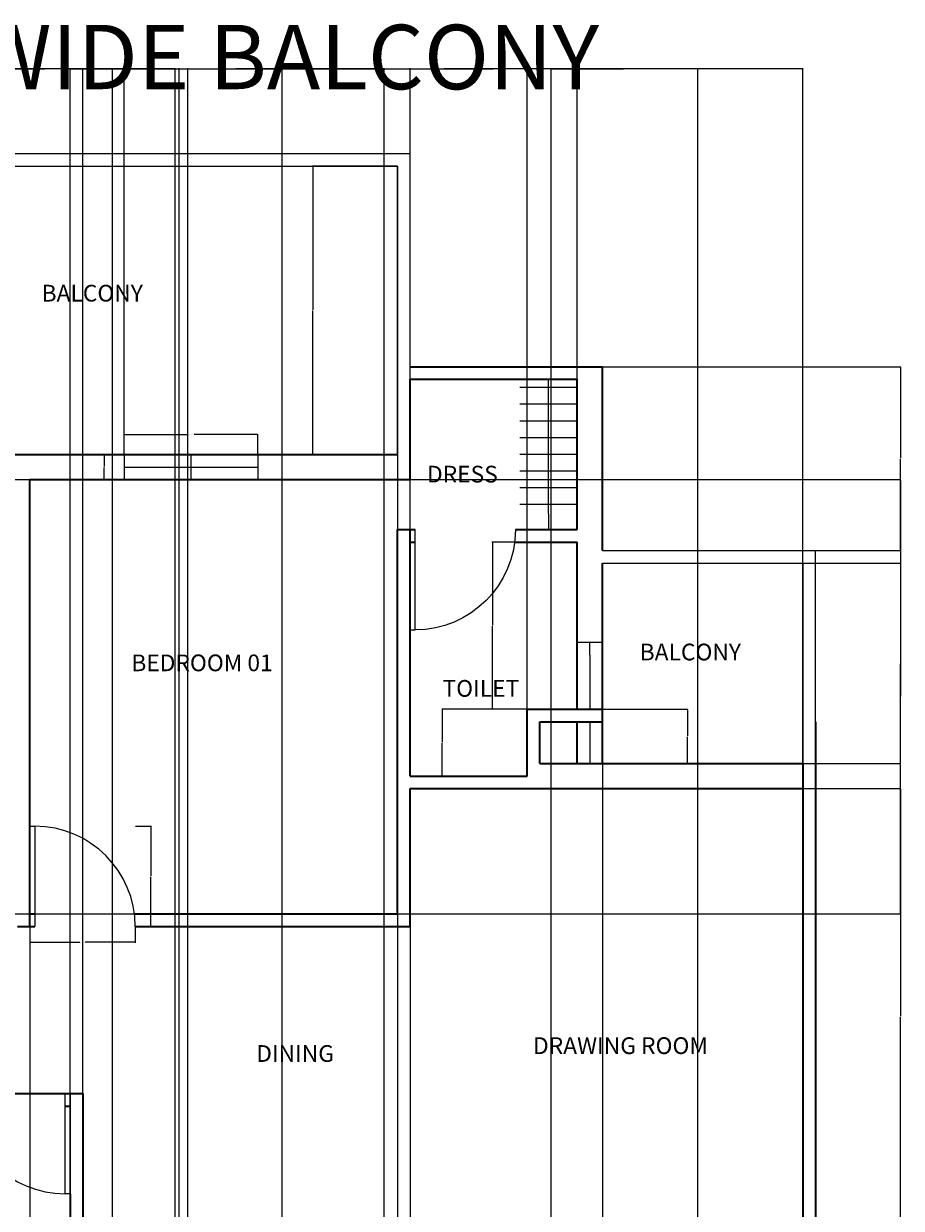
# Model space of a CAD drawing. Units: inches. Extents: x -83 to 475, y -99 to 539.
# Tile 3 of 3: x 160 to 475, y 114 to 539. Entities that reach past the tile are written whole.
import ezdxf

# ---------------------------------------------------------------- set-up
doc = ezdxf.new("R2010")
doc.units = ezdxf.units.IN
doc.header["$LTSCALE"] = 0.5
doc.header["$MEASUREMENT"] = 0
for name, color, linetype, lineweight in [('A-ANNO-DIMS', 2, 'Continuous', 18), ('A-ANNO-TEXT', 7, 'Continuous', 25), ('A-AREA-IDEN', 7, 'Continuous', 18), ('A-DOOR', 3, 'Continuous', 18), ('A-FURN', 8, 'Continuous', 13), ('A-GLAZ', 4, 'Continuous', 18), ('A-WALL', 7, 'Continuous', 35), ('A-WALL-PRPT', 7, 'Continuous', 25)]:
    doc.layers.add(name, color=color, linetype=linetype, lineweight=lineweight)
doc.styles.get("Standard").update_dxf_attribs({"font": 'arial.ttf'})
doc.dimstyles.get("Standard").update_dxf_attribs({"dimtxt": 0.18, "dimasz": 0.18, "dimexe": 0.18, "dimexo": 0.0625, "dimgap": 0.09, "dimtad": 0, "dimtih": 1, "dimtoh": 1, "dimdec": 4, "dimzin": 0, "dimdsep": 46, "dimtxsty": 'Standard', "dimcen": 0.09, "dimadec": 0, "dimazin": 0, "dimtfac": 1, "dimtdec": 4, "dimtofl": 0, "dimtmove": 0, "dimatfit": 3, "dimfxl": 1, "dimtolj": 1, "dimtzin": 0, "dimarcsym": 0})

# ---------------------------------------------------------------- blocks, each defined once
blk = doc.blocks.new('DOOR-SWING-36')
blk.add_lwpolyline([(1.78, 0), (0, 0), (0, 36.03), (1.78, 36.03)], close=True)
blk.add_arc((1.78, 0), 36, 0, 90)
blk = doc.blocks.new('WIN-48-TWO-LIGHT')
for p, q in [((0, 9), (0, 0)), ((24, 9), (24, 0)), ((48, 9), (48, 0)), ((0, 4.5), (48, 4.5))]:
    blk.add_line(p, q)
blk = doc.blocks.new('WIN-24')
for p, q in [((9, 24), (0, 24)), ((4.5, 19.41), (4.5, 24)), ((4.5, 19.41), (4.5, 0)), ((9, 0), (0, 0))]:
    blk.add_line(p, q)
blk = doc.blocks.new('WARDROBE-RAIL-48')
for p, q in [((2.64, 20.32), (2.64, 0)), ((8.64, 20.32), (8.64, 0)), ((14.64, 20.32), (14.64, 0)), ((20.64, 20.32), (20.64, 0)), ((26.64, 20.32), (26.64, 0)), ((32.64, 20.32), (32.64, 0)), ((38.64, 20.32), (38.64, 0)), ((44.64, 20.32), (44.64, 0)), ((48, 10.3), (0, 10.3))]:
    blk.add_line(p, q)
blk = doc.blocks.new('*D6')
at = {"layer": 'A-ANNO-DIMS', "color": 0, "lineweight": -2, "transparency": 16777216}
for p, q in [((162.04, 215.05), (162.04, 209.27)), ((199.82, 215.05), (199.82, 209.27)), ((162.22, 209.45), (180, 209.45)), ((199.64, 209.45), (181.87, 209.45))]:
    blk.add_line(p, q, dxfattribs=at)
at = {"layer": 'A-ANNO-DIMS', "color": 0, "transparency": 16777216}
for points in [[(162.22, 209.48), (162.22, 209.42), (162.04, 209.45)], [(199.64, 209.48), (199.64, 209.42), (199.82, 209.45)]]:
    blk.add_solid(points, dxfattribs=at)
at = {"layer": 'Defpoints', "color": 0, "transparency": 16777216}
for p in [(162.04, 215.11), (199.82, 215.11), (199.82, 209.45)]:
    blk.add_point(p, dxfattribs=at)
at = {"layer": 'A-ANNO-DIMS', "color": 0, "transparency": 16777216, "insert": (180.93, 209.45), "char_height": 0.18, "attachment_point": 5}
blk.add_mtext('\\A1;DOOR 38 TYP.', dxfattribs=at)
blk = doc.blocks.new('*D7')
at = {"layer": 'A-ANNO-DIMS', "color": 0, "lineweight": -2, "transparency": 16777216}
for p, q in [((199.89, 251.14), (205.67, 251.14)), ((205.49, 250.96), (205.49, 233.31)), ((205.49, 215.29), (205.49, 232.95)), ((199.89, 215.11), (205.67, 215.11))]:
    blk.add_line(p, q, dxfattribs=at)
at = {"layer": 'A-ANNO-DIMS', "color": 0, "transparency": 16777216}
for points in [[(205.46, 250.96), (205.52, 250.96), (205.49, 251.14)], [(205.46, 215.29), (205.52, 215.29), (205.49, 215.11)]]:
    blk.add_solid(points, dxfattribs=at)
at = {"layer": 'Defpoints', "color": 0, "transparency": 16777216}
for p in [(199.82, 251.14), (205.49, 251.14), (199.82, 215.11)]:
    blk.add_point(p, dxfattribs=at)
at = {"layer": 'A-ANNO-DIMS', "color": 0, "transparency": 16777216, "insert": (205.49, 233.13), "char_height": 0.18, "attachment_point": 5}
blk.add_mtext('\\A1;36 TYP.', dxfattribs=at)
blk = doc.blocks.new('*D8')
at = {"layer": 'A-ANNO-DIMS', "color": 0, "lineweight": -2, "transparency": 16777216}
for p, q in [((195.82, 384.62), (195.82, 391.94)), ((196, 391.76), (218.71, 391.76)), ((243.64, 391.76), (220.94, 391.76)), ((243.82, 384.62), (243.82, 391.94))]:
    blk.add_line(p, q, dxfattribs=at)
at = {"layer": 'A-ANNO-DIMS', "color": 0, "transparency": 16777216}
for points in [[(196, 391.79), (196, 391.73), (195.82, 391.76)], [(243.64, 391.79), (243.64, 391.73), (243.82, 391.76)]]:
    blk.add_solid(points, dxfattribs=at)
at = {"layer": 'Defpoints', "color": 0, "transparency": 16777216}
for p in [(243.82, 391.76), (195.82, 384.56), (243.82, 384.56)]:
    blk.add_point(p, dxfattribs=at)
at = {"layer": 'A-ANNO-DIMS', "color": 0, "transparency": 16777216, "insert": (219.82, 391.76), "char_height": 0.18, "attachment_point": 5}
blk.add_mtext('\\A1;WINDOW 48 TYP.', dxfattribs=at)
blk = doc.blocks.new('*D9')
at = {"layer": 'A-ANNO-DIMS', "color": 0, "lineweight": -2, "transparency": 16777216}
for p, q in [((195.76, 384.56), (188.44, 384.56)), ((188.62, 384.38), (188.62, 380.24)), ((188.62, 375.74), (188.62, 379.88)), ((195.76, 375.56), (188.44, 375.56))]:
    blk.add_line(p, q, dxfattribs=at)
at = {"layer": 'A-ANNO-DIMS', "color": 0, "transparency": 16777216}
for points in [[(188.59, 384.38), (188.65, 384.38), (188.62, 384.56)], [(188.59, 375.74), (188.65, 375.74), (188.62, 375.56)]]:
    blk.add_solid(points, dxfattribs=at)
at = {"layer": 'Defpoints', "color": 0, "transparency": 16777216}
for p in [(188.62, 384.56), (195.82, 384.56), (195.82, 375.56)]:
    blk.add_point(p, dxfattribs=at)
at = {"layer": 'A-ANNO-DIMS', "color": 0, "transparency": 16777216, "insert": (188.62, 380.06), "char_height": 0.18, "attachment_point": 5}
blk.add_mtext('\\A1;9 TYP.', dxfattribs=at)
blk = doc.blocks.new('*D15')
at = {"layer": 'A-ANNO-DIMS', "color": 0, "lineweight": -2, "transparency": 16777216}
for p, q in [((73.48, 492.61), (-83.14, 492.61)), ((-82.96, 492.43), (-82.96, 212.3)), ((-82.96, -68.21), (-82.96, 211.93)), ((214.1, -68.39), (-83.14, -68.39))]:
    blk.add_line(p, q, dxfattribs=at)
at = {"layer": 'A-ANNO-DIMS', "color": 0, "transparency": 16777216}
for points in [[(-82.99, 492.43), (-82.93, 492.43), (-82.96, 492.61)], [(-82.99, -68.21), (-82.93, -68.21), (-82.96, -68.39)]]:
    blk.add_solid(points, dxfattribs=at)
at = {"layer": 'Defpoints', "color": 0, "transparency": 16777216}
for p in [(-82.96, 492.61), (73.54, 492.61), (214.16, -68.39)]:
    blk.add_point(p, dxfattribs=at)
at = {"layer": 'A-ANNO-DIMS', "color": 0, "transparency": 16777216, "insert": (-82.96, 212.11), "char_height": 0.18, "attachment_point": 5}
blk.add_mtext('\\A1;561', dxfattribs=at)
blk = doc.blocks.new('*D16')
at = {"layer": 'A-ANNO-DIMS', "color": 0, "lineweight": -2, "transparency": 16777216}
for p, q in [((78.04, 488.05), (78.04, -99.07)), ((294.04, 488.05), (294.04, -99.07)), ((78.22, -98.89), (185.75, -98.89)), ((293.86, -98.89), (186.33, -98.89))]:
    blk.add_line(p, q, dxfattribs=at)
at = {"layer": 'A-ANNO-DIMS', "color": 0, "transparency": 16777216}
for points in [[(78.22, -98.86), (78.22, -98.92), (78.04, -98.89)], [(293.86, -98.86), (293.86, -98.92), (294.04, -98.89)]]:
    blk.add_solid(points, dxfattribs=at)
at = {"layer": 'Defpoints', "color": 0, "transparency": 16777216}
for p in [(78.04, 488.11), (294.04, 488.11), (294.04, -98.89)]:
    blk.add_point(p, dxfattribs=at)
at = {"layer": 'A-ANNO-DIMS', "color": 0, "transparency": 16777216, "insert": (186.04, -98.89), "char_height": 0.18, "attachment_point": 5}
blk.add_mtext('\\A1;216', dxfattribs=at)
blk = doc.blocks.new('*D17')
at = {"layer": 'A-ANNO-DIMS', "color": 0, "lineweight": -2, "transparency": 16777216}
for p, q in [((293.98, 488.11), (263.36, 488.11)), ((263.54, 487.93), (263.54, 436.55)), ((263.54, 384.79), (263.54, 436.18)), ((293.98, 384.61), (263.36, 384.61))]:
    blk.add_line(p, q, dxfattribs=at)
at = {"layer": 'A-ANNO-DIMS', "color": 0, "transparency": 16777216}
for points in [[(263.51, 487.93), (263.57, 487.93), (263.54, 488.11)], [(263.51, 384.79), (263.57, 384.79), (263.54, 384.61)]]:
    blk.add_solid(points, dxfattribs=at)
at = {"layer": 'Defpoints', "color": 0, "transparency": 16777216}
for p in [(263.54, 488.11), (294.04, 488.11), (294.04, 384.61)]:
    blk.add_point(p, dxfattribs=at)
at = {"layer": 'A-ANNO-DIMS', "color": 0, "transparency": 16777216, "insert": (263.54, 436.36), "char_height": 0.18, "attachment_point": 5}
blk.add_mtext('\\A1;103.5', dxfattribs=at)
blk = doc.blocks.new('*D20')
at = {"layer": 'A-ANNO-DIMS', "color": 0, "lineweight": -2, "transparency": 16777216}
for p, q in [((162.04, 375.55), (162.04, -99.07)), ((294.04, 357.55), (294.04, -99.07)), ((162.22, -98.89), (227.76, -98.89)), ((293.86, -98.89), (228.32, -98.89))]:
    blk.add_line(p, q, dxfattribs=at)
at = {"layer": 'A-ANNO-DIMS', "color": 0, "transparency": 16777216}
for points in [[(162.22, -98.86), (162.22, -98.92), (162.04, -98.89)], [(293.86, -98.86), (293.86, -98.92), (294.04, -98.89)]]:
    blk.add_solid(points, dxfattribs=at)
at = {"layer": 'Defpoints', "color": 0, "transparency": 16777216}
for p in [(162.04, 375.61), (294.04, 357.61), (294.04, -98.89)]:
    blk.add_point(p, dxfattribs=at)
at = {"layer": 'A-ANNO-DIMS', "color": 0, "transparency": 16777216, "insert": (228.04, -98.89), "char_height": 0.18, "attachment_point": 5}
blk.add_mtext('\\A1;132', dxfattribs=at)
blk = doc.blocks.new('*D21')
at = {"layer": 'A-ANNO-DIMS', "color": 0, "lineweight": -2, "transparency": 16777216}
for p, q in [((25.6, 375.61), (474.72, 375.61)), ((474.54, 375.43), (474.54, 297.8)), ((474.54, 219.79), (474.54, 297.43)), ((25.6, 219.61), (474.72, 219.61))]:
    blk.add_line(p, q, dxfattribs=at)
at = {"layer": 'A-ANNO-DIMS', "color": 0, "transparency": 16777216}
for points in [[(474.51, 375.43), (474.57, 375.43), (474.54, 375.61)], [(474.51, 219.79), (474.57, 219.79), (474.54, 219.61)]]:
    blk.add_solid(points, dxfattribs=at)
at = {"layer": 'Defpoints', "color": 0, "transparency": 16777216}
for p in [(25.54, 375.61), (474.54, 375.61), (25.54, 219.61)]:
    blk.add_point(p, dxfattribs=at)
at = {"layer": 'A-ANNO-DIMS', "color": 0, "transparency": 16777216, "insert": (474.54, 297.61), "char_height": 0.18, "attachment_point": 5}
blk.add_mtext('\\A1;156', dxfattribs=at)
blk = doc.blocks.new('*D22')
at = {"layer": 'A-ANNO-DIMS', "color": 0, "lineweight": -2, "transparency": 16777216}
for p, q in [((298.54, 411.68), (298.54, 523.29)), ((358.54, 411.68), (358.54, 523.29)), ((298.72, 523.11), (328.32, 523.11)), ((358.36, 523.11), (328.76, 523.11))]:
    blk.add_line(p, q, dxfattribs=at)
at = {"layer": 'A-ANNO-DIMS', "color": 0, "transparency": 16777216}
for points in [[(298.72, 523.14), (298.72, 523.08), (298.54, 523.11)], [(358.36, 523.14), (358.36, 523.08), (358.54, 523.11)]]:
    blk.add_solid(points, dxfattribs=at)
at = {"layer": 'Defpoints', "color": 0, "transparency": 16777216}
for p in [(358.54, 523.11), (298.54, 411.61), (358.54, 411.61)]:
    blk.add_point(p, dxfattribs=at)
at = {"layer": 'A-ANNO-DIMS', "color": 0, "transparency": 16777216, "insert": (328.54, 523.11), "char_height": 0.18, "attachment_point": 5}
blk.add_mtext('\\A1;60', dxfattribs=at)
blk = doc.blocks.new('*D23')
at = {"layer": 'A-ANNO-DIMS', "color": 0, "lineweight": -2, "transparency": 16777216}
for p, q in [((367.6, 416.11), (474.72, 416.11)), ((474.54, 415.93), (474.54, 383.3)), ((474.54, 350.29), (474.54, 382.93)), ((367.6, 350.11), (474.72, 350.11))]:
    blk.add_line(p, q, dxfattribs=at)
at = {"layer": 'A-ANNO-DIMS', "color": 0, "transparency": 16777216}
for points in [[(474.51, 415.93), (474.57, 415.93), (474.54, 416.11)], [(474.51, 350.29), (474.57, 350.29), (474.54, 350.11)]]:
    blk.add_solid(points, dxfattribs=at)
at = {"layer": 'Defpoints', "color": 0, "transparency": 16777216}
for p in [(367.54, 416.11), (474.54, 416.11), (367.54, 350.11)]:
    blk.add_point(p, dxfattribs=at)
at = {"layer": 'A-ANNO-DIMS', "color": 0, "transparency": 16777216, "insert": (474.54, 383.11), "char_height": 0.18, "attachment_point": 5}
blk.add_mtext('\\A1;66', dxfattribs=at)
blk = doc.blocks.new('*D24')
at = {"layer": 'A-ANNO-DIMS', "color": 0, "lineweight": -2, "transparency": 16777216}
for p, q in [((358.48, 353.11), (327.86, 353.11)), ((328.04, 352.93), (328.04, 323.3)), ((328.04, 293.29), (328.04, 322.93)), ((358.48, 293.11), (327.86, 293.11))]:
    blk.add_line(p, q, dxfattribs=at)
at = {"layer": 'A-ANNO-DIMS', "color": 0, "transparency": 16777216}
for points in [[(328.01, 352.93), (328.07, 352.93), (328.04, 353.11)], [(328.01, 293.29), (328.07, 293.29), (328.04, 293.11)]]:
    blk.add_solid(points, dxfattribs=at)
at = {"layer": 'Defpoints', "color": 0, "transparency": 16777216}
for p in [(328.04, 353.11), (358.54, 353.11), (358.54, 293.11)]:
    blk.add_point(p, dxfattribs=at)
at = {"layer": 'A-ANNO-DIMS', "color": 0, "transparency": 16777216, "insert": (328.04, 323.11), "char_height": 0.18, "attachment_point": 5}
blk.add_mtext('\\A1;60', dxfattribs=at)
blk = doc.blocks.new('*D25')
at = {"layer": 'A-ANNO-DIMS', "color": 0, "lineweight": -2, "transparency": 16777216}
for p, q in [((298.54, 269.18), (298.54, 523.29)), ((340.54, 269.18), (340.54, 523.29)), ((298.72, 523.11), (319.32, 523.11)), ((340.36, 523.11), (319.76, 523.11))]:
    blk.add_line(p, q, dxfattribs=at)
at = {"layer": 'A-ANNO-DIMS', "color": 0, "transparency": 16777216}
for points in [[(298.72, 523.14), (298.72, 523.08), (298.54, 523.11)], [(340.36, 523.14), (340.36, 523.08), (340.54, 523.11)]]:
    blk.add_solid(points, dxfattribs=at)
at = {"layer": 'Defpoints', "color": 0, "transparency": 16777216}
for p in [(340.54, 523.11), (298.54, 269.11), (340.54, 269.11)]:
    blk.add_point(p, dxfattribs=at)
at = {"layer": 'A-ANNO-DIMS', "color": 0, "transparency": 16777216, "insert": (319.54, 523.11), "char_height": 0.18, "attachment_point": 5}
blk.add_mtext('\\A1;42', dxfattribs=at)
blk = doc.blocks.new('*D26')
at = {"layer": 'A-ANNO-DIMS', "color": 0, "lineweight": -2, "transparency": 16777216}
for p, q in [((340.48, 293.11), (309.86, 293.11)), ((310.04, 292.93), (310.04, 281.29)), ((310.04, 269.29), (310.04, 280.93)), ((340.48, 269.11), (309.86, 269.11))]:
    blk.add_line(p, q, dxfattribs=at)
at = {"layer": 'A-ANNO-DIMS', "color": 0, "transparency": 16777216}
for points in [[(310.01, 292.93), (310.07, 292.93), (310.04, 293.11)], [(310.01, 269.29), (310.07, 269.29), (310.04, 269.11)]]:
    blk.add_solid(points, dxfattribs=at)
at = {"layer": 'Defpoints', "color": 0, "transparency": 16777216}
for p in [(310.04, 293.11), (340.54, 293.11), (340.54, 269.11)]:
    blk.add_point(p, dxfattribs=at)
at = {"layer": 'A-ANNO-DIMS', "color": 0, "transparency": 16777216, "insert": (310.04, 281.11), "char_height": 0.18, "attachment_point": 5}
blk.add_mtext('\\A1;24', dxfattribs=at)
blk = doc.blocks.new('*D27')
at = {"layer": 'A-ANNO-DIMS', "color": 0, "lineweight": -2, "transparency": 16777216}
for p, q in [((367.54, 345.55), (367.54, -99.07)), ((439.54, 345.55), (439.54, -99.07)), ((367.72, -98.89), (403.32, -98.89)), ((439.36, -98.89), (403.76, -98.89))]:
    blk.add_line(p, q, dxfattribs=at)
at = {"layer": 'A-ANNO-DIMS', "color": 0, "transparency": 16777216}
for points in [[(367.72, -98.86), (367.72, -98.92), (367.54, -98.89)], [(439.36, -98.86), (439.36, -98.92), (439.54, -98.89)]]:
    blk.add_solid(points, dxfattribs=at)
at = {"layer": 'Defpoints', "color": 0, "transparency": 16777216}
for p in [(367.54, 345.61), (439.54, 345.61), (439.54, -98.89)]:
    blk.add_point(p, dxfattribs=at)
at = {"layer": 'A-ANNO-DIMS', "color": 0, "transparency": 16777216, "insert": (403.54, -98.89), "char_height": 0.18, "attachment_point": 5}
blk.add_mtext('\\A1;72', dxfattribs=at)
blk = doc.blocks.new('*D28')
at = {"layer": 'A-ANNO-DIMS', "color": 0, "lineweight": -2, "transparency": 16777216}
for p, q in [((439.6, 345.61), (474.72, 345.61)), ((474.54, 345.43), (474.54, 309.79)), ((474.54, 273.79), (474.54, 309.43)), ((439.6, 273.61), (474.72, 273.61))]:
    blk.add_line(p, q, dxfattribs=at)
at = {"layer": 'A-ANNO-DIMS', "color": 0, "transparency": 16777216}
for points in [[(474.51, 345.43), (474.57, 345.43), (474.54, 345.61)], [(474.51, 273.79), (474.57, 273.79), (474.54, 273.61)]]:
    blk.add_solid(points, dxfattribs=at)
at = {"layer": 'Defpoints', "color": 0, "transparency": 16777216}
for p in [(439.54, 345.61), (474.54, 345.61), (439.54, 273.61)]:
    blk.add_point(p, dxfattribs=at)
at = {"layer": 'A-ANNO-DIMS', "color": 0, "transparency": 16777216, "insert": (474.54, 309.61), "char_height": 0.18, "attachment_point": 5}
blk.add_mtext('\\A1;72', dxfattribs=at)
blk = doc.blocks.new('*D35')
at = {"layer": 'A-ANNO-DIMS', "color": 0, "lineweight": -2, "transparency": 16777216}
for p, q in [((21.04, 18.68), (21.04, 523.29)), ((214.16, 18.68), (214.16, 523.29)), ((21.22, 523.11), (117.15, 523.11)), ((213.98, 523.11), (118.05, 523.11))]:
    blk.add_line(p, q, dxfattribs=at)
at = {"layer": 'A-ANNO-DIMS', "color": 0, "transparency": 16777216}
for points in [[(21.22, 523.14), (21.22, 523.08), (21.04, 523.11)], [(213.98, 523.14), (213.98, 523.08), (214.16, 523.11)]]:
    blk.add_solid(points, dxfattribs=at)
at = {"layer": 'Defpoints', "color": 0, "transparency": 16777216}
for p in [(214.16, 523.11), (21.04, 18.61), (214.16, 18.61)]:
    blk.add_point(p, dxfattribs=at)
at = {"layer": 'A-ANNO-DIMS', "color": 0, "transparency": 16777216, "insert": (117.6, 523.11), "char_height": 0.18, "attachment_point": 5}
blk.add_mtext('\\A1;193.12', dxfattribs=at)
blk = doc.blocks.new('*D41')
at = {"layer": 'A-ANNO-DIMS', "color": 0, "lineweight": -2, "transparency": 16777216}
for p, q in [((349.16, 51.68), (349.16, 523.29)), ((401.76, 51.68), (401.76, 523.29)), ((349.34, 523.11), (375.13, 523.11)), ((401.58, 523.11), (375.78, 523.11))]:
    blk.add_line(p, q, dxfattribs=at)
at = {"layer": 'A-ANNO-DIMS', "color": 0, "transparency": 16777216}
for points in [[(349.34, 523.14), (349.34, 523.08), (349.16, 523.11)], [(401.58, 523.14), (401.58, 523.08), (401.76, 523.11)]]:
    blk.add_solid(points, dxfattribs=at)
at = {"layer": 'Defpoints', "color": 0, "transparency": 16777216}
for p in [(401.76, 523.11), (349.16, 51.61), (401.76, 51.61)]:
    blk.add_point(p, dxfattribs=at)
at = {"layer": 'A-ANNO-DIMS', "color": 0, "transparency": 16777216, "insert": (375.46, 523.11), "char_height": 0.18, "attachment_point": 5}
blk.add_mtext('\\A1;52.6', dxfattribs=at)
blk = doc.blocks.new('*D43')
at = {"layer": 'A-ANNO-DIMS', "color": 0, "lineweight": -2, "transparency": 16777216}
for p, q in [((180.98, 101.18), (180.98, 523.29)), ((439.54, 83.2), (439.54, 523.29)), ((181.16, 523.11), (309.8, 523.11)), ((439.36, 523.11), (310.73, 523.11))]:
    blk.add_line(p, q, dxfattribs=at)
at = {"layer": 'A-ANNO-DIMS', "color": 0, "transparency": 16777216}
for points in [[(181.16, 523.14), (181.16, 523.08), (180.98, 523.11)], [(439.36, 523.14), (439.36, 523.08), (439.54, 523.11)]]:
    blk.add_solid(points, dxfattribs=at)
at = {"layer": 'Defpoints', "color": 0, "transparency": 16777216}
for p in [(439.54, 523.11), (180.98, 101.11), (439.54, 83.14)]:
    blk.add_point(p, dxfattribs=at)
at = {"layer": 'A-ANNO-DIMS', "color": 0, "transparency": 16777216, "insert": (310.26, 523.11), "char_height": 0.18, "attachment_point": 5}
blk.add_mtext('\\A1;258.56', dxfattribs=at)
blk = doc.blocks.new('*D44')
at = {"layer": 'A-ANNO-DIMS', "color": 0, "lineweight": -2, "transparency": 16777216}
for p, q in [((439.6, 264.61), (474.72, 264.61)), ((474.54, 264.43), (474.54, 183.05)), ((474.54, 101.29), (474.54, 182.68)), ((401.22, 101.11), (474.72, 101.11))]:
    blk.add_line(p, q, dxfattribs=at)
at = {"layer": 'A-ANNO-DIMS', "color": 0, "transparency": 16777216}
for points in [[(474.51, 264.43), (474.57, 264.43), (474.54, 264.61)], [(474.51, 101.29), (474.57, 101.29), (474.54, 101.11)]]:
    blk.add_solid(points, dxfattribs=at)
at = {"layer": 'Defpoints', "color": 0, "transparency": 16777216}
for p in [(439.54, 264.61), (474.54, 264.61), (401.16, 101.11)]:
    blk.add_point(p, dxfattribs=at)
at = {"layer": 'A-ANNO-DIMS', "color": 0, "transparency": 16777216, "insert": (474.54, 182.86), "char_height": 0.18, "attachment_point": 5}
blk.add_mtext('\\A1;163.5', dxfattribs=at)
blk = doc.blocks.new('*D45')
at = {"layer": 'A-ANNO-DIMS', "color": 0, "lineweight": -2, "transparency": 16777216}
for p, q in [((298.54, 264.55), (298.54, -99.07)), ((439.54, 264.55), (439.54, -99.07)), ((298.72, -98.89), (368.78, -98.89)), ((439.36, -98.89), (369.3, -98.89))]:
    blk.add_line(p, q, dxfattribs=at)
at = {"layer": 'A-ANNO-DIMS', "color": 0, "transparency": 16777216}
for points in [[(298.72, -98.86), (298.72, -98.92), (298.54, -98.89)], [(439.36, -98.86), (439.36, -98.92), (439.54, -98.89)]]:
    blk.add_solid(points, dxfattribs=at)
at = {"layer": 'Defpoints', "color": 0, "transparency": 16777216}
for p in [(298.54, 264.61), (439.54, 264.61), (439.54, -98.89)]:
    blk.add_point(p, dxfattribs=at)
at = {"layer": 'A-ANNO-DIMS', "color": 0, "transparency": 16777216, "insert": (369.04, -98.89), "char_height": 0.18, "attachment_point": 5}
blk.add_mtext('\\A1;141', dxfattribs=at)
blk = doc.blocks.new('*D47')
at = {"layer": 'A-ANNO-DIMS', "color": 0, "lineweight": -2, "transparency": 16777216}
for p, q in [((98.66, -45.82), (98.66, 523.29)), ((191.66, -45.82), (191.66, 523.29)), ((98.84, 523.11), (144.94, 523.11)), ((191.48, 523.11), (145.38, 523.11))]:
    blk.add_line(p, q, dxfattribs=at)
at = {"layer": 'A-ANNO-DIMS', "color": 0, "transparency": 16777216}
for points in [[(98.84, 523.14), (98.84, 523.08), (98.66, 523.11)], [(191.48, 523.14), (191.48, 523.08), (191.66, 523.11)]]:
    blk.add_solid(points, dxfattribs=at)
at = {"layer": 'Defpoints', "color": 0, "transparency": 16777216}
for p in [(191.66, 523.11), (98.66, -45.89), (191.66, -45.89)]:
    blk.add_point(p, dxfattribs=at)
at = {"layer": 'A-ANNO-DIMS', "color": 0, "transparency": 16777216, "insert": (145.16, 523.11), "char_height": 0.18, "attachment_point": 5}
blk.add_mtext('\\A1;93', dxfattribs=at)
blk = doc.blocks.new('*D48')
at = {"layer": 'A-ANNO-DIMS', "color": 0, "lineweight": -2, "transparency": 16777216}
for p, q in [((215.66, -63.82), (215.66, 523.29)), ((289.16, -63.82), (289.16, 523.29)), ((215.84, 523.11), (252.09, 523.11)), ((288.98, 523.11), (252.73, 523.11))]:
    blk.add_line(p, q, dxfattribs=at)
at = {"layer": 'A-ANNO-DIMS', "color": 0, "transparency": 16777216}
for points in [[(215.84, 523.14), (215.84, 523.08), (215.66, 523.11)], [(288.98, 523.14), (288.98, 523.08), (289.16, 523.11)]]:
    blk.add_solid(points, dxfattribs=at)
at = {"layer": 'Defpoints', "color": 0, "transparency": 16777216}
for p in [(289.16, 523.11), (215.66, -63.89), (289.16, -63.89)]:
    blk.add_point(p, dxfattribs=at)
at = {"layer": 'A-ANNO-DIMS', "color": 0, "transparency": 16777216, "insert": (252.41, 523.11), "char_height": 0.18, "attachment_point": 5}
blk.add_mtext('\\A1;73.5', dxfattribs=at)
blk = doc.blocks.new('*D53')
at = {"layer": 'A-ANNO-DIMS', "color": 0, "lineweight": -2, "transparency": 16777216}
for p, q in [((139.54, 384.68), (139.54, 523.29)), ((195.82, 384.62), (195.82, 523.29)), ((139.72, 523.11), (167.29, 523.11)), ((195.64, 523.11), (168.08, 523.11))]:
    blk.add_line(p, q, dxfattribs=at)
at = {"layer": 'A-ANNO-DIMS', "color": 0, "transparency": 16777216}
for points in [[(139.72, 523.14), (139.72, 523.08), (139.54, 523.11)], [(195.64, 523.14), (195.64, 523.08), (195.82, 523.11)]]:
    blk.add_solid(points, dxfattribs=at)
at = {"layer": 'Defpoints', "color": 0, "transparency": 16777216}
for p in [(195.82, 523.11), (139.54, 384.61), (195.82, 384.56)]:
    blk.add_point(p, dxfattribs=at)
at = {"layer": 'A-ANNO-DIMS', "color": 0, "transparency": 16777216, "insert": (167.68, 523.11), "char_height": 0.18, "attachment_point": 5}
blk.add_mtext('\\A1;56.28', dxfattribs=at)
blk = doc.blocks.new('*D54')
at = {"layer": 'A-ANNO-DIMS', "color": 0, "lineweight": -2, "transparency": 16777216}
for p, q in [((367.6, 293.11), (398.22, 293.11)), ((398.04, 292.93), (398.04, 283.55)), ((398.04, 273.79), (398.04, 283.18)), ((367.6, 273.61), (398.22, 273.61))]:
    blk.add_line(p, q, dxfattribs=at)
at = {"layer": 'A-ANNO-DIMS', "color": 0, "transparency": 16777216}
for points in [[(398.01, 292.93), (398.07, 292.93), (398.04, 293.11)], [(398.01, 273.79), (398.07, 273.79), (398.04, 273.61)]]:
    blk.add_solid(points, dxfattribs=at)
at = {"layer": 'Defpoints', "color": 0, "transparency": 16777216}
for p in [(367.54, 293.11), (367.54, 273.61), (398.04, 273.61)]:
    blk.add_point(p, dxfattribs=at)
at = {"layer": 'A-ANNO-DIMS', "color": 0, "transparency": 16777216, "insert": (398.04, 283.36), "char_height": 0.18, "attachment_point": 5}
blk.add_mtext('\\A1;19.5', dxfattribs=at)
blk = doc.blocks.new('*D58')
at = {"layer": 'A-ANNO-DIMS', "color": 0, "lineweight": -2, "transparency": 16777216}
for p, q in [((218.66, -23.32), (218.66, 523.29)), ((252.52, -23.32), (252.52, 523.29)), ((218.84, 523.11), (235.2, 523.11)), ((252.34, 523.11), (235.98, 523.11))]:
    blk.add_line(p, q, dxfattribs=at)
at = {"layer": 'A-ANNO-DIMS', "color": 0, "transparency": 16777216}
for points in [[(218.84, 523.14), (218.84, 523.08), (218.66, 523.11)], [(252.34, 523.14), (252.34, 523.08), (252.52, 523.11)]]:
    blk.add_solid(points, dxfattribs=at)
at = {"layer": 'Defpoints', "color": 0, "transparency": 16777216}
for p in [(252.52, 523.11), (218.66, -23.39), (252.52, -23.39)]:
    blk.add_point(p, dxfattribs=at)
at = {"layer": 'A-ANNO-DIMS', "color": 0, "transparency": 16777216, "insert": (235.59, 523.11), "char_height": 0.18, "attachment_point": 5}
blk.add_mtext('\\A1;33.86', dxfattribs=at)
blk = doc.blocks.new('*D61')
at = {"layer": 'A-ANNO-DIMS', "color": 0, "lineweight": -2, "transparency": 16777216}
for p, q in [((176.48, 96.68), (176.48, 523.29)), ((214.16, 96.68), (214.16, 523.29)), ((176.66, 523.11), (194.93, 523.11)), ((213.98, 523.11), (195.71, 523.11))]:
    blk.add_line(p, q, dxfattribs=at)
at = {"layer": 'A-ANNO-DIMS', "color": 0, "transparency": 16777216}
for points in [[(176.66, 523.14), (176.66, 523.08), (176.48, 523.11)], [(213.98, 523.14), (213.98, 523.08), (214.16, 523.11)]]:
    blk.add_solid(points, dxfattribs=at)
at = {"layer": 'Defpoints', "color": 0, "transparency": 16777216}
for p in [(214.16, 523.11), (176.48, 96.61), (214.16, 96.61)]:
    blk.add_point(p, dxfattribs=at)
at = {"layer": 'A-ANNO-DIMS', "color": 0, "transparency": 16777216, "insert": (195.32, 523.11), "char_height": 0.18, "attachment_point": 5}
blk.add_mtext('\\A1;37.68', dxfattribs=at)
blk = doc.blocks.new('*D62')
at = {"layer": 'A-ANNO-DIMS', "color": 0, "lineweight": -2, "transparency": 16777216}
for p, q in [((174.61, 155.11), (174.79, 155.11)), ((174.7, 155.02), (174.7, 155.2)), ((133.97, 114.38), (149.11, 129.53)), ((133.79, 114.38), (133.97, 114.38))]:
    blk.add_line(p, q, dxfattribs=at)
at = {"layer": 'A-ANNO-DIMS', "color": 0, "transparency": 16777216}
blk.add_solid([(149.09, 129.55), (149.13, 129.51), (149.24, 129.66)], dxfattribs=at)
at = {"layer": 'Defpoints', "color": 0, "transparency": 16777216}
for p in [(174.7, 155.11), (149.24, 129.66)]:
    blk.add_point(p, dxfattribs=at)
at = {"layer": 'A-ANNO-DIMS', "color": 0, "transparency": 16777216, "insert": (133.29, 114.38), "char_height": 0.18, "attachment_point": 5}
blk.add_mtext('\\A1;6X R36', dxfattribs=at)

msp = doc.modelspace()

# ---------------------------------------------------------------- linework, layer by layer
at = {"layer": 'A-DOOR'}
msp.add_line((174.697, 119.114), (174.697, 155.114), dxfattribs=at)
msp.add_lwpolyline([(176.481, 155.114), (176.481, 119.086), (174.697, 119.086), (174.697, 150.614)], dxfattribs=at)
msp.add_arc((174.697, 155.114), 36, 180, 270, dxfattribs=at)
at = {"layer": 'A-FURN'}
msp.add_line((348.216, 363.243), (348.216, 357.593), dxfattribs=at)
at = {"layer": 'A-GLAZ'}
msp.add_line((363.04, 288.614), (363.04, 273.614), dxfattribs=at)
at = {"layer": 'A-WALL'}
for p, q in [((298.54, 416.114), (367.54, 416.114)), ((298.54, 416.114), (367.54, 416.114)), ((298.54, 416.114), (367.54, 416.114)), ((367.54, 350.114), (367.54, 416.114)), ((298.54, 411.614), (358.54, 411.614)), ((298.54, 375.614), (298.54, 411.614)), ((298.54, 375.614), (298.54, 411.614)), ((358.54, 357.614), (358.54, 411.614)), ((78.04, 384.614), (294.04, 384.614)), ((162.04, 215.114), (162.04, 375.614)), ((162.04, 375.614), (298.54, 375.614)), ((294.04, 219.614), (294.04, 357.614)), ((294.04, 357.614), (300.324, 357.614)), ((294.04, 219.614), (294.04, 357.614)), ((298.54, 269.114), (298.54, 357.614)), ((336.324, 357.614), (358.54, 357.614)), ((298.54, 353.114), (300.324, 353.114)), ((298.54, 269.114), (298.54, 353.114)), ((336.042, 353.114), (358.54, 353.114)), ((358.54, 293.114), (358.54, 353.114)), ((367.54, 273.614), (367.54, 345.614)), ((340.54, 269.114), (340.54, 293.114)), ((340.54, 293.114), (367.54, 293.114)), ((345.04, 288.614), (367.54, 288.614)), ((345.04, 273.614), (345.04, 288.614)), ((358.54, 273.614), (358.54, 288.614)), ((444.04, 288.614), (444.04, 47.114)), ((345.04, 273.614), (367.54, 273.614)), ((367.54, 273.614), (439.54, 273.614)), ((439.54, 273.614), (439.54, 264.614)), ((298.54, 269.114), (340.54, 269.114)), ((298.54, 219.614), (298.54, 264.614)), ((298.54, 264.614), (439.54, 264.614)), ((298.54, 215.114), (298.54, 264.614)), ((439.54, 264.614), (439.54, 215.114)), ((162.04, 219.614), (163.824, 219.614)), ((199.542, 219.614), (294.04, 219.614)), ((199.542, 219.614), (294.04, 219.614)), ((157.54, 215.114), (163.824, 215.114)), ((199.824, 215.114), (298.54, 215.114)), ((199.824, 215.114), (298.54, 215.114)), ((439.54, 215.114), (439.54, 47.114)), ((113.54, 155.114), (180.981, 155.114)), ((180.981, 155.114), (180.981, 101.114)), ((174.697, 150.614), (176.1, 150.614)), ((176.481, 119.086), (176.481, 96.614))]:
    msp.add_line(p, q, dxfattribs=at)
at = {"layer": 'A-WALL-PRPT'}
for p, q in [((73.54, 492.614), (298.54, 492.614)), ((298.54, 416.114), (298.54, 492.614)), ((78.04, 488.114), (294.04, 488.114)), ((294.04, 384.614), (294.04, 488.114)), ((294.04, 384.614), (294.04, 416.114)), ((367.54, 350.114), (444.04, 350.114)), ((444.04, 273.614), (444.04, 350.114)), ((367.54, 345.614), (439.54, 345.614)), ((439.54, 273.614), (439.54, 345.614))]:
    msp.add_line(p, q, dxfattribs=at)

# ---------------------------------------------------------------- block references
at = {"layer": 'A-DOOR', "extrusion": (0, 0, -1), "zscale": -1, "rotation": 180}
msp.add_blockref('DOOR-SWING-36', (-298.54, 357.614), dxfattribs=at)
at = {"layer": 'A-DOOR'}
msp.add_blockref('DOOR-SWING-36', (162.04, 215.114), dxfattribs=at)
at = {"layer": 'A-FURN', "rotation": 269.9999999999998}
msp.add_blockref('WARDROBE-RAIL-48', (337.911, 411.243), dxfattribs=at)
at = {"layer": 'A-GLAZ'}
for name, p in [('WIN-48-TWO-LIGHT', (195.824, 375.561)), ('WIN-24', (358.54, 293.114))]:
    msp.add_blockref(name, p, dxfattribs=at)

# ---------------------------------------------------------------- texts
at = {"layer": 'A-ANNO-TEXT', "insert": (-32.222, 538.87), "char_height": 23.10502, "attachment_point": 1}
msp.add_mtext_dynamic_manual_height_columns('3BHK WITH WIDE BALCONY', width=1678.41017, gutter_width=115.525, heights=[0], dxfattribs=at)
at = {"layer": 'A-AREA-IDEN'}
for s, p in [('BALCONY', (166.226, 439.514)), ('DRESS', (304.575, 374.541)), ('BALCONY', (380.935, 310.661)), ('BEDROOM 01', (198.435, 306.767)), ('TOILET', (310.145, 297.602)), ('DRAWING ROOM', (342.646, 169.319)), ('DINING', (243.268, 166.497))]:
    msp.add_text(s, height=6, dxfattribs=at).set_placement(p)

# ---------------------------------------------------------------- dimensions: what is measured, and where the dimension line sits
at = {"layer": 'A-ANNO-DIMS'}
for base, p1, p2, override, picture, middle in [((214.161, 523.114), (21.04, 18.614), (214.161, 18.614), {"dimdec": 2, "dimlfac": 1, "dimrnd": 0, "dimzin": 0, "dimdsep": 46, "dimlunit": 2}, '*D35', (117.601, 523.114)), ((191.661, 523.114), (98.661, -45.886), (191.661, -45.886), {"dimdec": 0, "dimlfac": 1, "dimrnd": 0, "dimzin": 0, "dimdsep": 46, "dimlunit": 2}, '*D47', (145.161, 523.114)), ((195.824, 523.114), (139.54, 384.614), (195.824, 384.561), {"dimdec": 2, "dimlfac": 1, "dimrnd": 0, "dimzin": 0, "dimdsep": 46, "dimlunit": 2}, '*D53', (167.682, 523.114)), ((214.161, 523.114), (176.481, 96.614), (214.161, 96.614), {"dimdec": 2, "dimlfac": 1, "dimrnd": 0, "dimzin": 0, "dimdsep": 46, "dimlunit": 2}, '*D61', (195.321, 523.114)), ((439.54, 523.114), (180.981, 101.114), (439.54, 83.142), {"dimdec": 2, "dimlfac": 1, "dimrnd": 0, "dimzin": 0, "dimdsep": 46, "dimlunit": 2}, '*D43', (310.26, 523.114)), ((289.161, 523.114), (215.661, -63.886), (289.161, -63.886), {"dimdec": 1, "dimlfac": 1, "dimrnd": 0, "dimzin": 0, "dimdsep": 46, "dimlunit": 2}, '*D48', (252.411, 523.114)), ((252.52, 523.114), (218.661, -23.386), (252.52, -23.386), {"dimdec": 2, "dimlfac": 1, "dimrnd": 0, "dimzin": 0, "dimdsep": 46, "dimlunit": 2}, '*D58', (235.591, 523.114)), ((358.54, 523.114), (298.54, 411.614), (358.54, 411.614), {"dimdec": 0, "dimlfac": 1, "dimrnd": 0, "dimzin": 0, "dimdsep": 46, "dimlunit": 2}, '*D22', (328.54, 523.114)), ((340.54, 523.114), (298.54, 269.114), (340.54, 269.114), {"dimdec": 0, "dimlfac": 1, "dimrnd": 0, "dimzin": 0, "dimdsep": 46, "dimlunit": 2}, '*D25', (319.54, 523.114)), ((401.756, 523.114), (349.161, 51.614), (401.756, 51.614), {"dimdec": 1, "dimlfac": 1, "dimrnd": 0, "dimzin": 0, "dimdsep": 46, "dimlunit": 2}, '*D41', (375.459, 523.114)), ((294.04, -98.886), (78.04, 488.114), (294.04, 488.114), {"dimdec": 0, "dimlfac": 1, "dimrnd": 0, "dimzin": 0, "dimdsep": 46, "dimlunit": 2}, '*D16', (186.04, -98.886)), ((294.04, -98.886), (162.04, 375.614), (294.04, 357.614), {"dimdec": 0, "dimlfac": 1, "dimrnd": 0, "dimzin": 0, "dimdsep": 46, "dimlunit": 2}, '*D20', (228.04, -98.886)), ((439.54, -98.886), (367.54, 345.614), (439.54, 345.614), {"dimdec": 0, "dimlfac": 1, "dimrnd": 0, "dimzin": 0, "dimdsep": 46, "dimlunit": 2}, '*D27', (403.54, -98.886)), ((439.54, -98.886), (298.54, 264.614), (439.54, 264.614), {"dimdec": 0, "dimlfac": 1, "dimrnd": 0, "dimzin": 0, "dimdsep": 46, "dimlunit": 2}, '*D45', (369.04, -98.886))]:
    dim = msp.add_linear_dim(base=base, p1=p1, p2=p2, dimstyle='Standard', override=override, dxfattribs=at)
    dim.commit()
    dim.dimension.update_dxf_attribs({"geometry": picture, "text_midpoint": middle})
for base, p1, p2, angle, override, picture, middle in [((-82.96, 492.614), (214.161, -68.386), (73.54, 492.614), 90, {"dimdec": 0, "dimlfac": 1, "dimrnd": 0, "dimzin": 0, "dimdsep": 46, "dimlunit": 2}, '*D15', (-82.96, 212.114)), ((263.54, 488.114), (294.04, 384.614), (294.04, 488.114), 90, {"dimdec": 1, "dimlfac": 1, "dimrnd": 0, "dimzin": 0, "dimdsep": 46, "dimlunit": 2}, '*D17', (263.54, 436.364)), ((474.54, 416.114), (367.54, 350.114), (367.54, 416.114), 90, {"dimdec": 0, "dimlfac": 1, "dimrnd": 0, "dimzin": 0, "dimdsep": 46, "dimlunit": 2}, '*D23', (474.54, 383.114)), ((474.54, 375.614), (25.54, 219.614), (25.54, 375.614), 90, {"dimdec": 0, "dimlfac": 1, "dimrnd": 0, "dimzin": 0, "dimdsep": 46, "dimlunit": 2}, '*D21', (474.54, 297.614)), ((328.04, 353.114), (358.54, 293.114), (358.54, 353.114), 90, {"dimdec": 0, "dimlfac": 1, "dimrnd": 0, "dimzin": 0, "dimdsep": 46, "dimlunit": 2}, '*D24', (328.04, 323.114)), ((474.54, 345.614), (439.54, 273.614), (439.54, 345.614), 90, {"dimdec": 0, "dimlfac": 1, "dimrnd": 0, "dimzin": 0, "dimdsep": 46, "dimlunit": 2}, '*D28', (474.54, 309.614)), ((310.04, 293.114), (340.54, 269.114), (340.54, 293.114), 90, {"dimdec": 0, "dimlfac": 1, "dimrnd": 0, "dimzin": 0, "dimdsep": 46, "dimlunit": 2}, '*D26', (310.04, 281.114)), ((398.04, 273.614), (367.54, 293.114), (367.54, 273.614), 269.99999, {"dimdec": 1, "dimlfac": 1, "dimrnd": 0, "dimzin": 0, "dimdsep": 46, "dimlunit": 2}, '*D54', (398.04, 283.364)), ((474.54, 264.614), (401.161, 101.114), (439.54, 264.614), 90, {"dimdec": 1, "dimlfac": 1, "dimrnd": 0, "dimzin": 0, "dimdsep": 46, "dimlunit": 2}, '*D44', (474.54, 182.864))]:
    dim = msp.add_linear_dim(base=base, p1=p1, p2=p2, angle=angle, dimstyle='Standard', override=override, dxfattribs=at)
    dim.commit()
    dim.dimension.update_dxf_attribs({"geometry": picture, "text_midpoint": middle})
for base, p1, p2, text, picture, middle in [((243.824, 391.761), (195.824, 384.561), (243.824, 384.561), 'WINDOW <> TYP.', '*D8', (219.824, 391.761)), ((199.824, 209.447), (162.04, 215.114), (199.824, 215.114), 'DOOR <> TYP.', '*D6', (180.932, 209.447))]:
    dim = msp.add_linear_dim(base=base, p1=p1, p2=p2, text=text, dimstyle='Standard', override={"dimdec": 0, "dimlfac": 1, "dimrnd": 0, "dimzin": 0, "dimdsep": 46, "dimlunit": 2}, dxfattribs=at)
    dim.commit()
    dim.dimension.update_dxf_attribs({"geometry": picture, "text_midpoint": middle})
for base, p1, p2, picture, middle in [((188.624, 384.561), (195.824, 375.561), (195.824, 384.561), '*D9', (188.624, 380.061)), ((205.492, 251.142), (199.824, 215.114), (199.824, 251.142), '*D7', (205.492, 233.128))]:
    dim = msp.add_linear_dim(base=base, p1=p1, p2=p2, angle=90, text='<> TYP.', dimstyle='Standard', override={"dimdec": 0, "dimlfac": 1, "dimrnd": 0, "dimzin": 0, "dimdsep": 46, "dimlunit": 2}, dxfattribs=at)
    dim.commit()
    dim.dimension.update_dxf_attribs({"geometry": picture, "text_midpoint": middle})
dim = msp.add_radius_dim(center=(174.697, 155.114), mpoint=(149.241, 129.658), text='6X <>', dimstyle='Standard', override={"dimdec": 0, "dimlfac": 1, "dimrnd": 0, "dimzin": 0, "dimdsep": 46, "dimlunit": 2}, dxfattribs=at)
dim.commit()
dim.dimension.update_dxf_attribs({"geometry": '*D62', "text_midpoint": (133.289, 114.384), "dimtype": 164})

doc.saveas('drawing.dxf')
